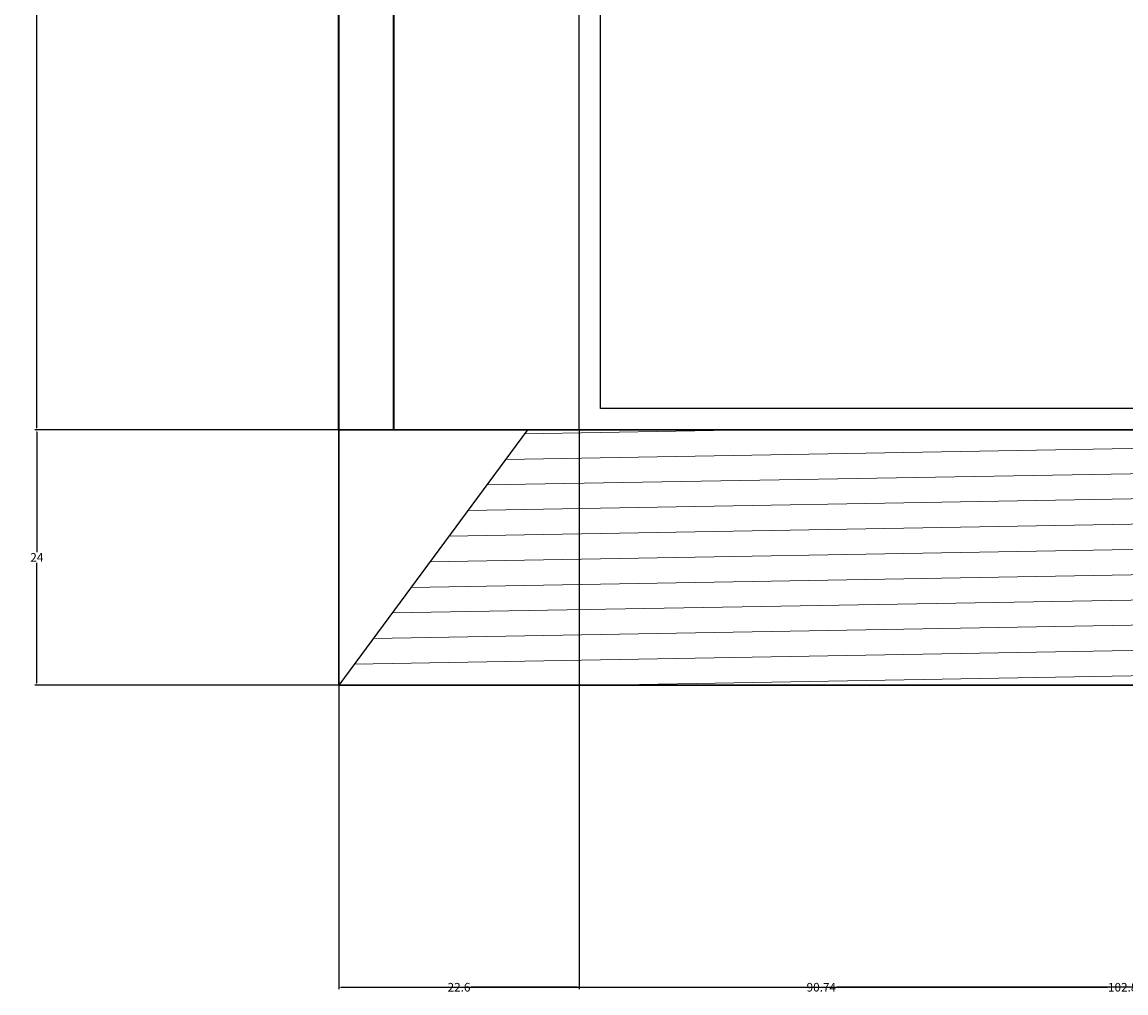
# Model space of a CAD drawing. Units: inches. Extents: x 69 to 650, y -16 to 573.
# Tile 1 of 26: x 70 to 174, y 35 to 126. Entities that reach past the tile are written whole.
import ezdxf

# ---------------------------------------------------------------- set-up
doc = ezdxf.new("R2010")
doc.units = ezdxf.units.IN
doc.header["$MEASUREMENT"] = 0
for name, color, linetype, lineweight in [('A-ANNO-DIMS', 2, 'Continuous', 18), ('A-DOOR', 3, 'Continuous', 25), ('A-FLOR-PATT', 252, 'Continuous', 13), ('A-FLOR-STRS', 7, 'Continuous', 25), ('A-WALL', 7, 'Continuous', 35), ('A-WALL-BASE', 7, 'Continuous', 30)]:
    doc.layers.add(name, color=color, linetype=linetype, lineweight=lineweight)
doc.styles.get("Standard").update_dxf_attribs({"font": 'arial.ttf'})
doc.dimstyles.get("Standard").update_dxf_attribs({"dimtxt": 0.8125, "dimasz": 0.18, "dimexe": 0.18, "dimexo": 0.0625, "dimgap": 0.09, "dimtad": 0, "dimtih": 1, "dimtoh": 1, "dimdec": 4, "dimzin": 0, "dimdsep": 46, "dimlunit": 4, "dimtxsty": 'Standard', "dimcen": 0.09, "dimadec": 0, "dimazin": 0, "dimtfac": 1, "dimtdec": 4, "dimtofl": 0, "dimtmove": 0, "dimatfit": 3, "dimfxl": 1, "dimtolj": 1, "dimtzin": 0, "dimarcsym": 0})

# ---------------------------------------------------------------- blocks, each defined once
blk = doc.blocks.new('*D19')
at = {"layer": 'A-ANNO-DIMS', "color": 0, "lineweight": -2, "transparency": 16777216}
for p, q in [((99.56, 471.72), (99.56, 572.74)), ((99.74, 572.56), (358.57, 572.56)), ((619.38, 572.56), (360.54, 572.56)), ((619.56, 87.99), (619.56, 572.74))]:
    blk.add_line(p, q, dxfattribs=at)
at = {"layer": 'A-ANNO-DIMS', "color": 0, "transparency": 16777216}
for points in [[(99.74, 572.59), (99.74, 572.53), (99.56, 572.56)], [(619.38, 572.59), (619.38, 572.53), (619.56, 572.56)]]:
    blk.add_solid(points, dxfattribs=at)
at = {"layer": 'Defpoints', "color": 0, "transparency": 16777216}
for p in [(619.56, 572.56), (99.56, 471.66), (619.56, 87.93)]:
    blk.add_point(p, dxfattribs=at)
at = {"layer": 'A-ANNO-DIMS', "color": 0, "transparency": 16777216, "insert": (359.56, 572.56), "char_height": 0.812, "attachment_point": 5}
blk.add_mtext('\\A1;520', dxfattribs=at)
blk = doc.blocks.new('*D21')
at = {"layer": 'A-ANNO-DIMS', "color": 0, "lineweight": -2, "transparency": 16777216}
for p, q in [((99.49, 87.93), (70.98, 87.93)), ((71.16, 87.75), (71.16, 76.43)), ((71.16, 64.11), (71.16, 75.43)), ((99.49, 63.93), (70.98, 63.93))]:
    blk.add_line(p, q, dxfattribs=at)
at = {"layer": 'A-ANNO-DIMS', "color": 0, "transparency": 16777216}
for points in [[(71.13, 87.75), (71.19, 87.75), (71.16, 87.93)], [(71.13, 64.11), (71.19, 64.11), (71.16, 63.93)]]:
    blk.add_solid(points, dxfattribs=at)
at = {"layer": 'Defpoints', "color": 0, "transparency": 16777216}
for p in [(71.16, 87.93), (99.56, 87.93), (99.56, 63.93)]:
    blk.add_point(p, dxfattribs=at)
at = {"layer": 'A-ANNO-DIMS', "color": 0, "transparency": 16777216, "insert": (71.16, 75.93), "char_height": 0.812, "attachment_point": 5}
blk.add_mtext('\\A1;24', dxfattribs=at)
blk = doc.blocks.new('*D22')
at = {"layer": 'A-ANNO-DIMS', "color": 0, "lineweight": -2, "transparency": 16777216}
for p, q in [((122.09, 187.88), (70.98, 187.88)), ((71.16, 187.7), (71.16, 138.41)), ((71.16, 88.11), (71.16, 137.4)), ((122.09, 87.93), (70.98, 87.93))]:
    blk.add_line(p, q, dxfattribs=at)
at = {"layer": 'A-ANNO-DIMS', "color": 0, "transparency": 16777216}
for points in [[(71.13, 187.7), (71.19, 187.7), (71.16, 187.88)], [(71.13, 88.11), (71.19, 88.11), (71.16, 87.93)]]:
    blk.add_solid(points, dxfattribs=at)
at = {"layer": 'Defpoints', "color": 0, "transparency": 16777216}
for p in [(71.16, 187.88), (122.16, 187.88), (122.16, 87.93)]:
    blk.add_point(p, dxfattribs=at)
at = {"layer": 'A-ANNO-DIMS', "color": 0, "transparency": 16777216, "insert": (71.16, 137.91), "char_height": 0.812, "attachment_point": 5}
blk.add_mtext('\\A1;99.95', dxfattribs=at)
blk = doc.blocks.new('*D26')
at = {"layer": 'A-ANNO-DIMS', "color": 0, "lineweight": -2, "transparency": 16777216}
for p, q in [((99.56, 87.87), (99.56, 35.35)), ((122.16, 87.87), (122.16, 35.35)), ((99.74, 35.53), (109.7, 35.53)), ((121.98, 35.53), (112.01, 35.53))]:
    blk.add_line(p, q, dxfattribs=at)
at = {"layer": 'A-ANNO-DIMS', "color": 0, "transparency": 16777216}
for points in [[(99.74, 35.56), (99.74, 35.5), (99.56, 35.53)], [(121.98, 35.56), (121.98, 35.5), (122.16, 35.53)]]:
    blk.add_solid(points, dxfattribs=at)
at = {"layer": 'Defpoints', "color": 0, "transparency": 16777216}
for p in [(99.56, 87.93), (122.16, 87.93), (122.16, 35.53)]:
    blk.add_point(p, dxfattribs=at)
at = {"layer": 'A-ANNO-DIMS', "color": 0, "transparency": 16777216, "insert": (110.86, 35.53), "char_height": 0.812, "attachment_point": 5}
blk.add_mtext('\\A1;22.6', dxfattribs=at)
blk = doc.blocks.new('*D27')
at = {"layer": 'A-ANNO-DIMS', "color": 0, "lineweight": -2, "transparency": 16777216}
for p, q in [((122.16, 87.87), (122.16, 35.35)), ((225, 87.87), (225, 35.35)), ((122.34, 35.53), (171.84, 35.53)), ((224.82, 35.53), (175.31, 35.53))]:
    blk.add_line(p, q, dxfattribs=at)
at = {"layer": 'A-ANNO-DIMS', "color": 0, "transparency": 16777216}
for points in [[(122.34, 35.56), (122.34, 35.5), (122.16, 35.53)], [(224.82, 35.56), (224.82, 35.5), (225, 35.53)]]:
    blk.add_solid(points, dxfattribs=at)
at = {"layer": 'Defpoints', "color": 0, "transparency": 16777216}
for p in [(122.16, 87.93), (225, 87.93), (225, 35.53)]:
    blk.add_point(p, dxfattribs=at)
at = {"layer": 'A-ANNO-DIMS', "color": 0, "transparency": 16777216, "insert": (173.58, 35.53), "char_height": 0.812, "attachment_point": 5}
blk.add_mtext('\\A1;102.84', dxfattribs=at)
blk = doc.blocks.new('*D35')
at = {"layer": 'A-ANNO-DIMS', "color": 0, "lineweight": -2, "transparency": 16777216}
for p, q in [((99.56, 243.87), (99.56, 35.35)), ((190.3, 243.87), (190.3, 35.35)), ((99.74, 35.53), (143.47, 35.53)), ((190.12, 35.53), (146.39, 35.53))]:
    blk.add_line(p, q, dxfattribs=at)
at = {"layer": 'A-ANNO-DIMS', "color": 0, "transparency": 16777216}
for points in [[(99.74, 35.56), (99.74, 35.5), (99.56, 35.53)], [(190.12, 35.56), (190.12, 35.5), (190.3, 35.53)]]:
    blk.add_solid(points, dxfattribs=at)
at = {"layer": 'Defpoints', "color": 0, "transparency": 16777216}
for p in [(99.56, 243.93), (190.3, 243.93), (190.3, 35.53)]:
    blk.add_point(p, dxfattribs=at)
at = {"layer": 'A-ANNO-DIMS', "color": 0, "transparency": 16777216, "insert": (144.93, 35.53), "char_height": 0.812, "attachment_point": 5}
blk.add_mtext('\\A1;90.74', dxfattribs=at)

msp = doc.modelspace()

# ---------------------------------------------------------------- hatches: boundary and pattern name
at = {"layer": 'A-FLOR-PATT'}
h = msp.add_hatch(dxfattribs=at)
h.set_pattern_fill('ANSI31', color=256, scale=19, angle=136)
h.paths.add_polyline_path([(232.9803, 87.93), (117.2878, 87.93), (99.556, 63.93), (240.241, 63.93)])

# ---------------------------------------------------------------- linework, layer by layer
at = {"layer": 'A-DOOR'}
for points in [[(122.1565, 174.2116), (224.9972, 174.2116), (224.9972, 87.93), (122.1565, 87.93)], [(124.1565, 172.2116), (222.9972, 172.2116), (222.9972, 89.93), (124.1565, 89.93)]]:
    msp.add_lwpolyline(points, close=True, dxfattribs=at)
at = {"layer": 'A-FLOR-STRS'}
msp.add_lwpolyline([(117.2878, 87.93), (99.556, 63.93)], dxfattribs=at)
at = {"layer": 'A-WALL'}
for p, q in [((99.556, 87.93), (99.556, 231.93)), ((104.6982, 231.93), (104.6982, 87.93))]:
    msp.add_line(p, q, dxfattribs=at)
at = {"layer": 'A-WALL-BASE'}
for p, q in [((99.556, 87.93), (463.7847, 87.93)), ((99.556, 87.93), (99.556, 63.93)), ((99.556, 63.93), (463.7847, 63.93))]:
    msp.add_line(p, q, dxfattribs=at)

# ---------------------------------------------------------------- dimensions: what is measured, and where the dimension line sits
at = {"layer": 'A-ANNO-DIMS'}
for base, p1, p2, override, picture, middle in [((619.555, 572.5573), (99.556, 471.6595), (619.555, 87.93), {"dimdec": 0, "dimlfac": 1, "dimrnd": 0, "dimzin": 0, "dimdsep": 46, "dimlunit": 2}, '*D19', (359.5555, 572.5573)), ((190.299, 35.53), (99.556, 243.93), (190.299, 243.93), {"dimdec": 2, "dimlfac": 1, "dimrnd": 0, "dimzin": 0, "dimdsep": 46, "dimlunit": 2}, '*D35', (144.9275, 35.53)), ((122.1565, 35.53), (99.556, 87.93), (122.1565, 87.93), {"dimdec": 1, "dimlfac": 1, "dimrnd": 0, "dimzin": 0, "dimdsep": 46, "dimlunit": 2}, '*D26', (110.8563, 35.53)), ((224.9972, 35.53), (122.1565, 87.93), (224.9972, 87.93), {"dimdec": 2, "dimlfac": 1, "dimrnd": 0, "dimzin": 0, "dimdsep": 46, "dimlunit": 2}, '*D27', (173.5769, 35.53))]:
    dim = msp.add_linear_dim(base=base, p1=p1, p2=p2, dimstyle='Standard', override=override, dxfattribs=at)
    dim.commit()
    dim.dimension.update_dxf_attribs({"geometry": picture, "text_midpoint": middle})
for base, p1, p2, override, picture, middle in [((71.156, 187.8805), (122.1565, 87.93), (122.1565, 187.8805), {"dimdec": 2, "dimlfac": 1, "dimrnd": 0, "dimzin": 0, "dimdsep": 46, "dimlunit": 2}, '*D22', (71.156, 137.9053)), ((71.156, 87.93), (99.556, 63.93), (99.556, 87.93), {"dimdec": 0, "dimlfac": 1, "dimrnd": 0, "dimzin": 0, "dimdsep": 46, "dimlunit": 2}, '*D21', (71.156, 75.93))]:
    dim = msp.add_linear_dim(base=base, p1=p1, p2=p2, angle=90, dimstyle='Standard', override=override, dxfattribs=at)
    dim.commit()
    dim.dimension.update_dxf_attribs({"geometry": picture, "text_midpoint": middle})

doc.saveas('drawing.dxf')
